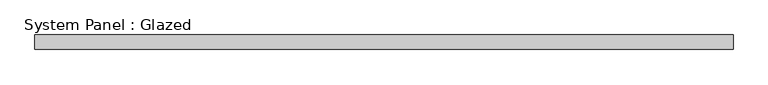
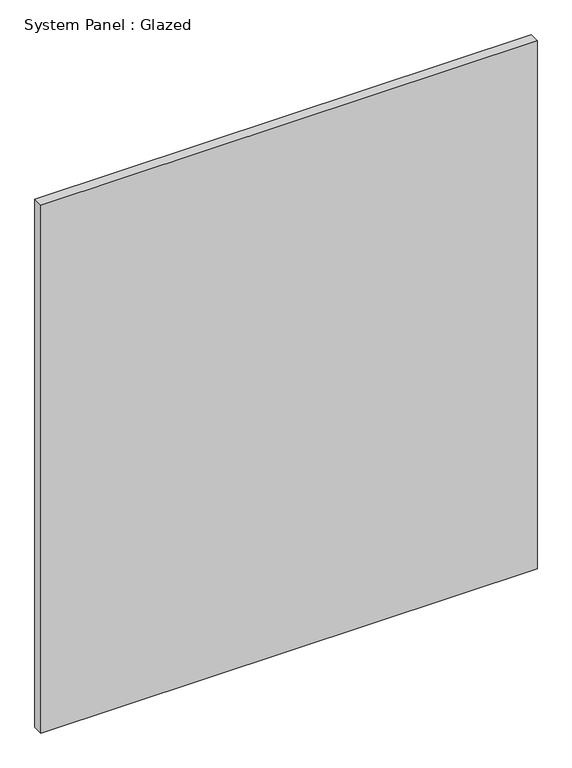
"""IFC4 building model written with IfcOpenShell, lengths in millimetres: plate geometry, System Panel : Glazed."""

from ifc_helpers import new_model, si_unit, origin, origin_with_axes, place, context, project, spatial, polyline, outline, extrude, source, transform, mapped, element, save


def system_panel_glazed_45b685ca(model_context):
    return source(origin(), model_context, "Body", "SweptSolid", [
        extrude(outline(polyline([(609.6, 19.05), (-609.6, 19.05), (-609.6, 44.45), (609.6, 44.45), (609.6, 19.05)])), origin_with_axes(), (0.0, 0.0, 1.0), 1371.6),
    ])


if __name__ == "__main__":
    model = new_model("IFC4")
    model_context = context("Model", 3, world=origin())
    ifc_project = project(units=[si_unit("LENGTHUNIT", "METRE", prefix="MILLI")], contexts=[model_context])
    site = spatial("IfcSite", under=ifc_project)
    building = spatial("IfcBuilding", under=site)
    placement = place(None, origin())
    system_panel_glazed_shape = system_panel_glazed_45b685ca(model_context)
    element("IfcPlate", 1, ObjectType="System Panel : Glazed", at=placement, inside=building, context=model_context, shape_type="MappedRepresentation", body=[
        mapped(system_panel_glazed_shape, transform((0.0, 0.0, 0.0), x_axis=(1.0, 0.0, 0.0), y_axis=(0.0, 1.0, 0.0), z_axis=(0.0, 0.0, 1.0))),
    ])
    save(model, "model.ifc")

# Revit data of these elements
# Type "System Panel : Glazed"
#   Construction Type Id = "GSP4R"
#   Analytic Construction = "1/8 in Pilkington single glazing"
#   Visual Light Transmittance = 0.9
#   Solar Heat Gain Coefficient = 0.86
#   Heat Transfer Coefficient (U) = 1.18115 BTU/(h·ft²·°F)
#   Define Thermal Properties by = 1
# Element 1 (IfcPlate, "System Panel : Glazed")
#   Materials on its faces: "Glass"
# Materials
#   "Glass": class "Glass", colour RGB 0 128 192, transparency 0.75, Description = "Soda Lime Glass", Cost = 0
